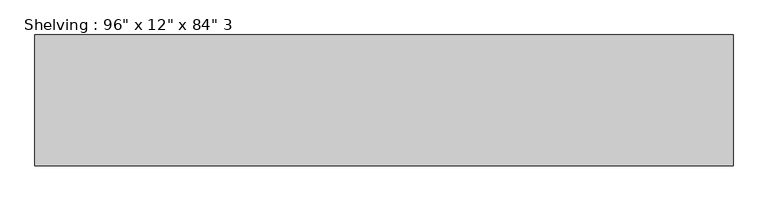
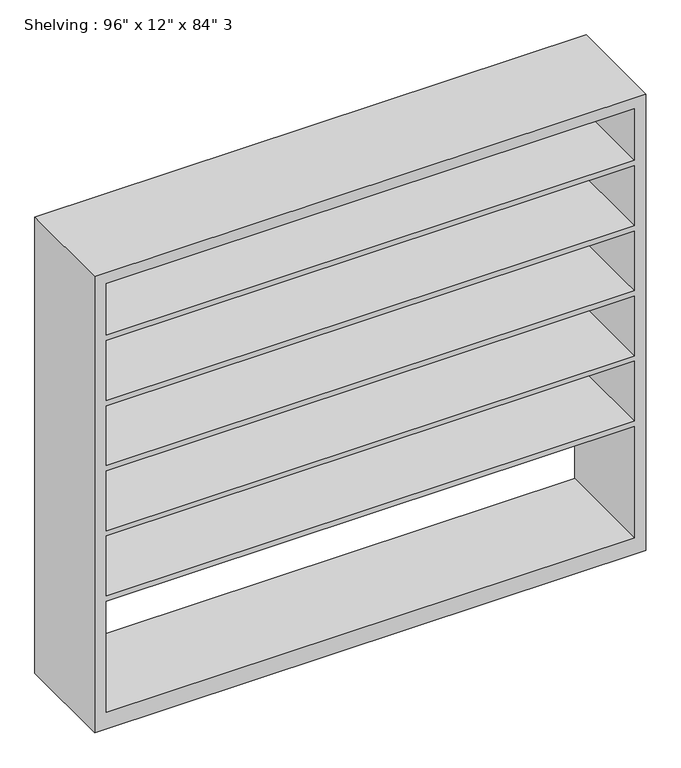
"""IFC4 building model written with IfcOpenShell, lengths in millimetres: furniture geometry."""

from ifc_helpers import new_model, si_unit, frame, origin, place, context, project, spatial, polyline, outline, extrude, source, transform, mapped, element, save


def furniture_57be741f(model_context):
    return source(origin(), model_context, "Body", "SweptSolid", [
        extrude(outline(polyline([(0.0, 1219.2), (2133.6, 1219.2), (2133.6, -1219.2), (0.0, -1219.2), (0.0, 1219.2)]), holes=[polyline([(2082.8, 1168.4), (1841.5, 1168.4), (1841.5, -1168.4), (2082.8, -1168.4), (2082.8, 1168.4)]), polyline([(76.2, 1168.4), (76.2, -1168.4), (596.9, -1168.4), (596.9, 1168.4), (76.2, 1168.4)]), polyline([(1231.9, -1168.4), (1511.3, -1168.4), (1511.3, 1168.4), (1231.9, 1168.4), (1231.9, -1168.4)]), polyline([(1816.1, 1168.4), (1536.7, 1168.4), (1536.7, -1168.4), (1816.1, -1168.4), (1816.1, 1168.4)]), polyline([(1206.5, 1168.4), (927.1, 1168.4), (927.1, -1168.4), (1206.5, -1168.4), (1206.5, 1168.4)]), polyline([(901.7, 1168.4), (622.3, 1168.4), (622.3, -1168.4), (901.7, -1168.4), (901.7, 1168.4)])]), frame((0.0, -533.4, 0.0), z_axis=(0.0, 1.0, 0.0), x_axis=(0.0, 0.0, 1.0)), (0.0, 0.0, 1.0), 457.2),
    ])


if __name__ == "__main__":
    model = new_model("IFC4")
    model_context = context("Model", 3, world=origin())
    ifc_project = project(units=[si_unit("LENGTHUNIT", "METRE", prefix="MILLI")], contexts=[model_context])
    site = spatial("IfcSite", under=ifc_project)
    building = spatial("IfcBuilding", under=site)
    placement = place(None, origin())
    furniture_shape = furniture_57be741f(model_context)
    element("IfcFurniture", 1, ObjectType="Shelving : 96\" x 12\" x 84\" 3", at=placement, inside=building, context=model_context, shape_type="MappedRepresentation", body=[
        mapped(furniture_shape, transform((0.0, 0.0, 0.0), x_axis=(1.0, 0.0, 0.0), y_axis=(0.0, 1.0, 0.0), z_axis=(0.0, 0.0, 1.0))),
    ])
    save(model, "model.ifc")

# Revit data of these elements
# Type "Shelving : 96\" x 12\" x 84\" 3"
#   Assembly Code = "E2020200"
#   Depth = 1' - 6"
#   Height = 7' - 0"
#   Width = 8' - 0"
#   Shelving Unit Material = Laminate, Ivory, Matte
#   Default Elevation = 0
# Element 1 (IfcFurniture, "Shelving : 96\" x 12\" x 84\" 3")
#   Materials on its faces: "Laminate, Ivory, Matte"
# Materials
#   "Laminate, Ivory, Matte": class "Plastic", colour RGB 247 247 239, transparency 0, Description = "Plastic Laminate - Ivory, Matte", Cost = 0
